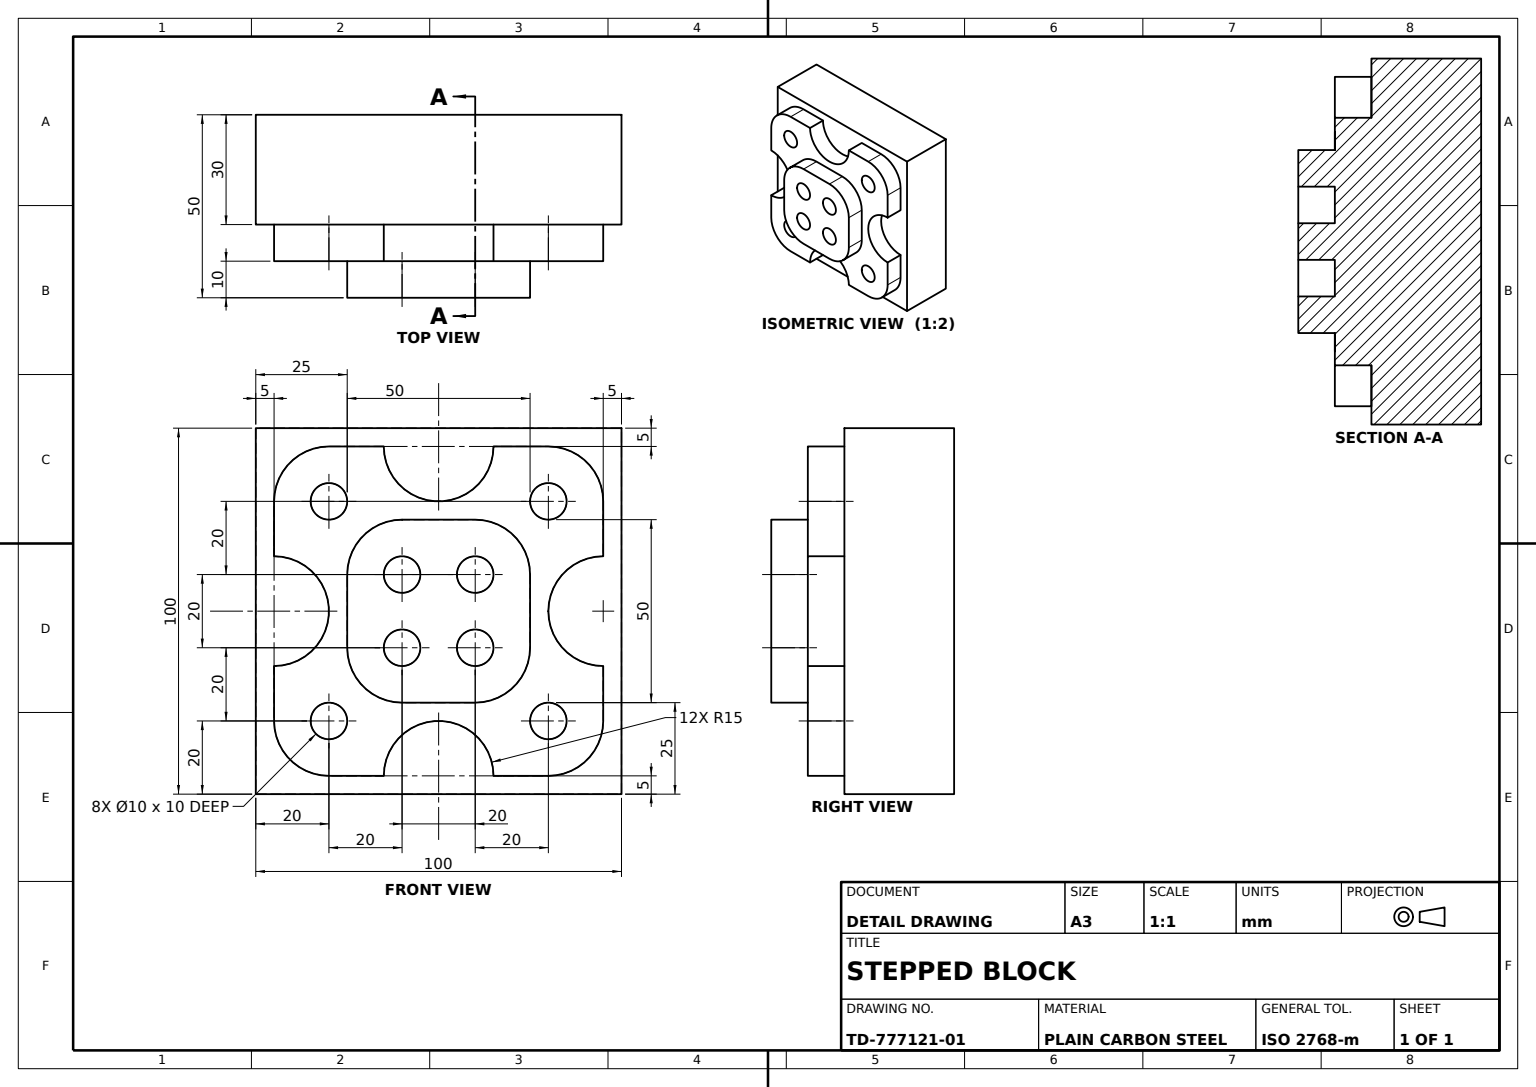
SolidWorks part; units mm, degrees
material "Plain Carbon Steel"
ref_plane "Front Plane" through (0, 0, 0) normal (0, 0, 1) x (1, 0, 0)
ref_plane "Top Plane" through (0, 0, 0) normal (0, 1, 0) x (1, 0, 0)
ref_plane "Right Plane" through (0, 0, 0) normal (1, 0, 0) x (0, 0, -1)
sketch "Base Block Sketch" plane through (0, 0, 0) normal (0, 0, 1) x (1, 0, 0)
  line L0 (0, 0) -> (0, -100)
  line L1 (0, -100) -> (100, -100)
  line L2 (100, -100) -> (100, 0)
  line L3 (100, 0) -> (0, 0)
  dimension "D1" = 100
extrude "Base Block 100x100x30" add sketch "Base Block Sketch" along normal blind 30
sketch "Flange Plate Sketch" plane through (0, 0, 30) normal (0, 0, 1) x (1, 0, 0)
  line L0 (5, -65) -> (5, -80)
  line L1 (20, -5) -> (35, -5)
  line L2 (5, -20) -> (5, -35)
  line L3 (20, -95) -> (35, -95)
  line L4 (95, -20) -> (95, -35)
  line L5 (65, -5) -> (80, -5)
  line L6 (95, -65) -> (95, -80)
  line L7 (65, -95) -> (80, -95)
  line L8 (100, 0) -> (0, 0) construction
  line L9 (100, -100) -> (100, 0) construction
  line L10 (0, -100) -> (100, -100) construction
  line L11 (0, 0) -> (0, -100) construction
  arc A0 (5, -65) -> (5, -35) centre (5, -50) ccw
  arc A1 (95, -35) -> (95, -65) centre (95, -50) ccw
  arc A2 (65, -95) -> (35, -95) centre (50, -95) ccw
  arc A3 (35, -5) -> (65, -5) centre (50, -5) ccw
  arc A4 (20, -95) -> (5, -80) centre (20, -80) cw
  arc A5 (80, -95) -> (95, -80) centre (80, -80) ccw
  arc A6 (95, -20) -> (80, -5) centre (80, -20) ccw
  arc A7 (20, -5) -> (5, -20) centre (20, -20) ccw
  dimension "D5" = 30
  dimension "D6" = 30
  dimension "D7" = 30
  dimension "D8" = 15
  dimension "D9" = 15
  dimension "D1" = 5
  dimension "D2" = 5
  dimension "D3" = 5
  dimension "D4" = 5
  dimension "D10" = 50
  dimension "D11" = 50
extrude "Flange Plate" add sketch "Flange Plate Sketch" along normal blind 10
sketch "Centre Boss Sketch" plane through (0, 0, 40) normal (0, 0, 1) x (1, 0, 0)
  line L7 (25, -40) -> (25, -60)
  line L8 (40, -75) -> (60, -75)
  line L9 (75, -40) -> (75, -60)
  line L10 (40, -25) -> (60, -25)
  line L11 (95, -80) -> (95, -65) construction
  line L12 (65, -95) -> (80, -95) construction
  arc A0 (40, -25) -> (25, -40) centre (40, -40) ccw
  arc A3 (25, -60) -> (40, -75) centre (40, -60) ccw
  arc A4 (75, -40) -> (60, -25) centre (60, -40) ccw
  arc A6 (60, -75) -> (75, -60) centre (60, -60) ccw
  dimension "D1" = 30
  dimension "D2" = 15
  dimension "D3" = 20
  dimension "D4" = 30
  dimension "D5" = 70
  dimension "D6" = 20
extrude "Centre Boss" add sketch "Centre Boss Sketch" along normal blind 10
sketch "Boss Holes Sketch" plane through (0, 0, 50) normal (0, 0, 1) x (1, 0, 0)
  circle A0 centre (40, -40) radius 5
  circle A1 centre (60, -40) radius 5
  circle A2 centre (60, -60) radius 5
  circle A3 centre (40, -60) radius 5
  dimension "D1" = 10
  dimension "D2" = 10
  dimension "D3" = 10
  dimension "D4" = 10
  dimension "D5" = 10
extrude "Boss Holes 4xØ10" cut sketch "Boss Holes Sketch" against normal blind 10
sketch "Flange Holes Sketch" plane through (0, 0, 40) normal (0, 0, 1) x (1, 0, 0)
  circle A0 centre (20, -20) radius 5
  circle A1 centre (80, -20) radius 5
  circle A2 centre (80, -80) radius 5
  circle A3 centre (20, -80) radius 5
  dimension "D1" = 10
  dimension "D2" = 10
  dimension "D3" = 10
  dimension "D4" = 10
  dimension "D5" = 10
extrude "Flange Holes 4xØ10" cut sketch "Flange Holes Sketch" against normal blind 10
